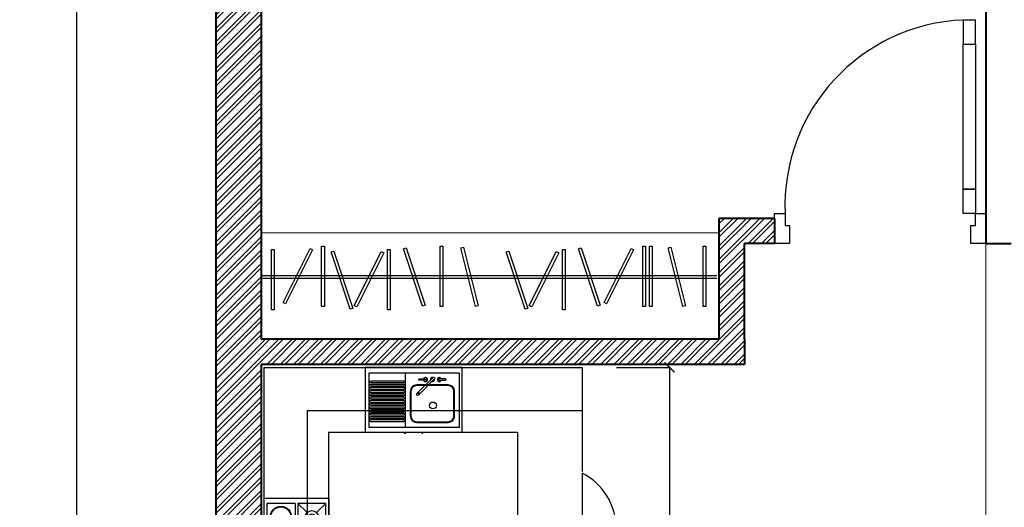
# Model space of a CAD drawing. Units: inches. Extents: x 528 to 2520, y -151 to 1354.
# Tile 30 of 41: x 2119 to 2315, y 635 to 731. Entities that reach past the tile are written whole.
import ezdxf

# ---------------------------------------------------------------- set-up
doc = ezdxf.new("R2010")
doc.units = ezdxf.units.IN
doc.header["$MEASUREMENT"] = 0
for name, color, linetype, lineweight in [('A-ANNO-DIMS', 2, 'Continuous', 18), ('A-Door', 150, 'Continuous', 25), ('A-ELEV-PROJ', 8, 'Continuous', 13), ('A-FLOR-CASE', 11, 'Continuous', 20), ('A-WALL-PATT', 6, 'Continuous', 13), ('walls', 7, 'Continuous', 40)]:
    doc.layers.add(name, color=color, linetype=linetype, lineweight=lineweight)
for name, color, linetype in [('ESYA', 11, 'Continuous'), ('HID', 11, 'Continuous'), ('NT', 1, 'Continuous'), ('TEFRIS', 11, 'Continuous')]:
    doc.layers.add(name, color=color, linetype=linetype)
doc.styles.get("Standard").update_dxf_attribs({"font": 'arial.ttf'})
doc.dimstyles.get("Standard").update_dxf_attribs({"dimtxt": 6, "dimasz": 2, "dimexe": 0.18, "dimexo": 0.0625, "dimgap": 0.09, "dimtad": 0, "dimtih": 1, "dimtoh": 1, "dimdec": 1, "dimzin": 0, "dimdsep": 46, "dimlunit": 3, "dimtxsty": 'Standard', "dimblk": 'ARCHTICK', "dimcen": 0.09, "dimadec": 0, "dimazin": 0, "dimtfac": 1, "dimtdec": 1, "dimtofl": 0, "dimtmove": 0, "dimatfit": 3, "dimfxl": 1, "dimtolj": 1, "dimtzin": 0, "dimarcsym": 0})

# ---------------------------------------------------------------- blocks, each defined once
blk = doc.blocks.new('A$C7DB75F4D')
at = {"layer": 'A-Door'}
for points in [[(625, 740), (625, 660), (665, 660), (665, 740)], [(625, 180), (625, 660), (665, 660), (665, 180)], [(625, 100), (625, 180), (665, 180), (665, 100)], [(35, 100), (35, 60), (50, 60), (50, 50), (50, 0), (0, 0), (0, 100)], [(665, 100), (700, 100), (700, 0), (650, 0), (650, 50), (650, 60), (665, 60)]]:
    blk.add_lwpolyline(points, close=True, dxfattribs=at)
at = {"layer": 'NT'}
blk.add_arc((650, 125), 615.5, 92.3278, 182.3278, dxfattribs=at)
blk = doc.blocks.new('A$C41BE763B')
at = {"layer": 'HID'}
for p, q in [((3.395, 0.2532), (0, 0.2532)), ((3.395, 0.2332), (0, 0.2332))]:
    blk.add_line(p, q, dxfattribs=at)
for points in [[(0.0983, 0.45), (0.0983, 0), (0.0775, 0), (0.0775, 0.45)], [(0.3834, 0.447), (0.1822, 0.0445), (0.1636, 0.0538), (0.3648, 0.4563)], [(0.4716, 0.4734), (0.4716, 0.0234), (0.4508, 0.0234), (0.4508, 0.4734)], [(0.9617, 0.45), (0.9617, 0), (0.941, 0), (0.941, 0.45)], [(1.0809, 0.4606), (1.2232, 0.0337), (1.2035, 0.0271), (1.0612, 0.454)], [(1.3547, 0.4734), (1.3547, 0.0234), (1.3339, 0.0234), (1.3339, 0.4734)], [(1.5084, 0.466), (1.6175, 0.0294), (1.5974, 0.0244), (1.4882, 0.4609)], [(2.2657, 0.45), (2.2657, 0), (2.2449, 0), (2.2449, 0.45)], [(2.3849, 0.4606), (2.5272, 0.0337), (2.5075, 0.0271), (2.3652, 0.454)], [(2.7757, 0.447), (2.5745, 0.0445), (2.5559, 0.0538), (2.7572, 0.4563)], [(2.8639, 0.4734), (2.8639, 0.0234), (2.8432, 0.0234), (2.8432, 0.4734)], [(2.9139, 0.4734), (2.9139, 0.0234), (2.8932, 0.0234), (2.8932, 0.4734)], [(3.0533, 0.466), (3.1624, 0.0294), (3.1423, 0.0244), (3.0332, 0.4609)], [(3.3139, 0.4734), (3.3139, 0.0234), (3.2932, 0.0234), (3.2932, 0.4734)], [(0.5408, 0.4372), (0.6831, 0.0103), (0.6634, 0.0037), (0.5211, 0.4306)], [(0.914, 0.4236), (0.7128, 0.0211), (0.6942, 0.0304), (0.8954, 0.4329)], [(1.8448, 0.4372), (1.9871, 0.0103), (1.9674, 0.0037), (1.8251, 0.4306)], [(2.218, 0.4236), (2.0167, 0.0211), (1.9981, 0.0304), (2.1994, 0.4329)]]:
    blk.add_lwpolyline(points, close=True, dxfattribs=at)
blk = doc.blocks.new('AR365L')
blk.add_line((0, 0.0995), (0.61, 0.0995))
blk.add_lwpolyline([(0, 0), (0, 0.68), (0.61, 0.68), (0.61, 0)], close=True)
blk = doc.blocks.new('FIRIN1')
at = {"layer": 'ESYA'}
for p, q in [((0.2875, -0.05), (0.2875, -0.3006)), ((0.3983, -0.1319), (0.3125, -0.05)), ((0.575, -0.05), (0.4892, -0.1319)), ((0.3983, -0.2187), (0.3125, -0.3006)), ((0.575, -0.3006), (0.4892, -0.2187)), ((0.2875, -0.3006), (0.025, -0.3006)), ((0.025, -0.3244), (0.1108, -0.4063)), ((0.2017, -0.4063), (0.2875, -0.3244)), ((0.3983, -0.4063), (0.3125, -0.3244)), ((0.575, -0.3244), (0.4892, -0.4063)), ((0.025, -0.575), (0.1108, -0.4931)), ((0.2017, -0.4931), (0.2875, -0.575)), ((0.3983, -0.4931), (0.3125, -0.575)), ((0.575, -0.575), (0.4892, -0.4931))]:
    blk.add_line(p, q, dxfattribs=at)
blk.add_lwpolyline([(0, 0), (0.6, 0), (0.6, -0.6), (0, -0.6)], close=True, dxfattribs=at)
for points in [[(0.2875, -0.05), (0.025, -0.05), (0.025, -0.3006)], [(0.3125, -0.05), (0.3125, -0.3006), (0.575, -0.3006)], [(0.575, -0.3006), (0.575, -0.05), (0.3125, -0.05)], [(0.2875, -0.575), (0.2875, -0.3244), (0.025, -0.3244)], [(0.025, -0.3244), (0.025, -0.575)], [(0.3125, -0.575), (0.3125, -0.3244), (0.575, -0.3244)], [(0.3125, -0.575), (0.575, -0.575), (0.575, -0.3244)], [(0.025, -0.575), (0.2875, -0.575)]]:
    blk.add_lwpolyline(points, dxfattribs=at)
for centre, radius in [((0.1562, -0.1753), 0.0986), ((0.1562, -0.1753), 0.0936), ((0.4438, -0.1753), 0.0597), ((0.4438, -0.1753), 0.0294), ((0.1562, -0.4497), 0.0492), ((0.1562, -0.4497), 0.0242), ((0.4438, -0.4497), 0.0398), ((0.4438, -0.4497), 0.0196)]:
    blk.add_circle(centre, radius, dxfattribs=at)
blk = doc.blocks.new('ncvn')
for p, q in [((77868.38, -4466.7), (77868.38, -4520.7)), ((77949.38, -4466.7), (77868.38, -4466.7)), ((77949.38, -4520.7), (77949.38, -4466.7))]:
    blk.add_line(p, q)
at = {"layer": 'TEFRIS'}
for p, q in [((77783.66, -4466.69), (77783.66, -4763.38)), ((77783.66, -4466.69), (78049.52, -4466.69)), ((78049.52, -4466.69), (78049.52, -4553.55)), ((77901.95, -4516.62), (77901.95, -4471.62)), ((77819.66, -4502.83), (77819.66, -4759.23)), ((77819.66, -4502.83), (78049.52, -4502.83)), ((77837.66, -4520.83), (77837.66, -4704.71)), ((77837.66, -4520.83), (77995.52, -4520.83)), ((77868.38, -4520.7), (77949.38, -4520.7)), ((77995.52, -4520.83), (77995.52, -4642.99)), ((78049.52, -4554.99), (78049.52, -4625.66)), ((78049.52, -4625.66), (77995.83, -4625.66)), ((77783.66, -4704.71), (77837.66, -4704.71))]:
    blk.add_line(p, q, dxfattribs=at)
for points in [[(77868.38, -4466.7), (77868.38, -4520.7), (77949.38, -4520.7), (77949.38, -4466.7)], [(77871.35, -4471.62), (77871.35, -4516.62), (77946.95, -4516.62), (77946.95, -4471.62)]]:
    blk.add_lwpolyline(points, close=True, dxfattribs=at)
for points in [[(77911.5, -4488.58), (77925.04, -4475.05, -1), (77926.25, -4476.26), (77912.72, -4489.8, -1)], [(77905.95, -4486.73), (77905.95, -4507.22, 0.414214), (77911.35, -4512.62), (77937.55, -4512.62, 0.414214), (77942.95, -4507.22), (77942.95, -4486.73, 0.414214), (77937.55, -4481.33), (77911.35, -4481.33, 0.414214)], [(77906.49, -4486.73), (77906.49, -4507.22, 0.414214), (77911.35, -4512.08), (77937.55, -4512.08, 0.414214), (77942.41, -4507.22), (77942.41, -4486.73, 0.414214), (77937.55, -4481.87), (77911.35, -4481.87, 0.414214)], [(77913.54, -4476.29), (77919.71, -4476.29, -0.563183), (77919.71, -4477.44), (77913.54, -4477.44, -1)], [(77935.33, -4476.29), (77929.17, -4476.29, 0.563183), (77929.17, -4477.44), (77935.33, -4477.44, 1)]]:
    blk.add_lwpolyline(points, format="xyb", close=True, dxfattribs=at)
for points in [[(77873.15, -4477.92), (77900.15, -4477.92, -1), (77900.15, -4479.72), (77873.15, -4479.72, -1), (77873.15, -4477.92)], [(77873.15, -4480.62), (77900.15, -4480.62, -1), (77900.15, -4482.42), (77873.15, -4482.42, -1), (77873.15, -4480.62)], [(77873.15, -4483.32), (77900.15, -4483.32, -1), (77900.15, -4485.12), (77873.15, -4485.12, -1), (77873.15, -4483.32)], [(77873.15, -4486.02), (77900.15, -4486.02, -1), (77900.15, -4487.82), (77873.15, -4487.82, -1), (77873.15, -4486.02)], [(77873.15, -4488.72), (77900.15, -4488.72, -1), (77900.15, -4490.52), (77873.15, -4490.52, -1), (77873.15, -4488.72)], [(77873.15, -4491.42), (77900.15, -4491.42, -1), (77900.15, -4493.22), (77873.15, -4493.22, -1), (77873.15, -4491.42)], [(77873.15, -4494.12), (77900.15, -4494.12, -1), (77900.15, -4495.92), (77873.15, -4495.92, -1), (77873.15, -4494.12)], [(77873.15, -4496.82), (77900.15, -4496.82, -1), (77900.15, -4498.62), (77873.15, -4498.62, -1), (77873.15, -4496.82)], [(77873.15, -4499.52), (77900.15, -4499.52, -1), (77900.15, -4501.32), (77873.15, -4501.32, -1), (77873.15, -4499.52)], [(77873.15, -4502.22), (77900.15, -4502.22, -1), (77900.15, -4504.02), (77873.15, -4504.02, -1), (77873.15, -4502.22)], [(77873.15, -4504.92), (77900.15, -4504.92, -1), (77900.15, -4506.72), (77873.15, -4506.72, -1), (77873.15, -4504.92)], [(77873.15, -4507.62), (77900.15, -4507.62, -1), (77900.15, -4509.42), (77873.15, -4509.42, -1), (77873.15, -4507.62)], [(77873.15, -4510.32), (77900.15, -4510.32, -1), (77900.15, -4512.12), (77873.15, -4512.12, -1), (77873.15, -4510.32)]]:
    blk.add_lwpolyline(points, format="xyb", dxfattribs=at)
for points in [[(77901.23, -4520.7), (77901.23, -4521.6), (77902.13, -4521.6), (77902.13, -4520.7)], [(77915.63, -4520.7), (77915.63, -4521.6), (77916.53, -4521.6), (77916.53, -4520.7)]]:
    blk.add_lwpolyline(points, dxfattribs=at)
for centre, radius in [((77913.01, -4488.3), 0.571), ((77924.89, -4498.48), 2.86)]:
    blk.add_circle(centre, radius, dxfattribs=at)
for centre, radius, start, end in [((77918.69, -4476.87), 1.71, 199.47122, 160.52878), ((77924.44, -4476.87), 1.71, 75, 195), ((77930.19, -4476.87), 1.71, 19.47122, 340.52878), ((77924.44, -4476.87), 1.71, 255, 15), ((78026.22, -4601.26), 51.8, 233.6588, 63.26709)]:
    blk.add_arc(centre, radius, start, end, dxfattribs=at)
at = {"layer": 'TEFRIS', "xscale": 90, "yscale": 90, "zscale": 90}
blk.add_blockref('FIRIN1', (77783.76, -4575.88), dxfattribs=at)
at = {"layer": 'TEFRIS', "xscale": 90, "yscale": 90, "zscale": 90, "rotation": 90}
blk.add_blockref('AR365L', (77848.22, -4760.91), dxfattribs=at)
blk = doc.blocks.new('_ArchTick')
at = {"color": 0, "linetype": 'ByBlock', "const_width": 0.15}
blk.add_lwpolyline([(-0.5, -0.5), (0.5, 0.5)], dxfattribs=at)
blk = doc.blocks.new('*D60')
at = {"layer": 'A-ANNO-DIMS', "color": 0, "lineweight": -2, "transparency": 16777216}
for p, q in [((2237.62, 662.36), (2248.32, 662.36)), ((2248.14, 662.36), (2248.14, 630.29)), ((2248.14, 591.82), (2248.14, 623.9)), ((2237.62, 591.82), (2248.32, 591.82))]:
    blk.add_line(p, q, dxfattribs=at)
at = {"layer": 'Defpoints', "color": 0, "transparency": 16777216}
for p in [(2237.56, 662.36), (2248.14, 662.36), (2237.56, 591.82)]:
    blk.add_point(p, dxfattribs=at)
at = {"layer": 'A-ANNO-DIMS', "color": 0, "lineweight": -2, "transparency": 16777216, "xscale": 2, "yscale": 2, "zscale": 2}
for p, rotation in [((2248.14, 662.36), 90), ((2248.14, 591.82), 270)]:
    blk.add_blockref('_ArchTick', p, dxfattribs=dict(at, rotation=rotation))
at = {"layer": 'A-ANNO-DIMS', "color": 0, "transparency": 16777216, "insert": (2248.14, 627.09), "char_height": 6, "attachment_point": 5}
blk.add_mtext('\\A1;KITCHEN COUNTER 5\'-10 1/2" TYP.', dxfattribs=at)
blk = doc.blocks.new('*D95')
at = {"layer": 'A-ANNO-DIMS', "color": 0, "lineweight": -2, "transparency": 16777216}
for p, q in [((2157.95, 897.94), (2130.18, 897.94)), ((2130.36, 897.94), (2130.36, 632.59)), ((2130.36, 360.94), (2130.36, 626.29)), ((2157.95, 360.94), (2130.18, 360.94))]:
    blk.add_line(p, q, dxfattribs=at)
at = {"layer": 'Defpoints', "color": 0, "transparency": 16777216}
for p in [(2130.36, 897.94), (2158.01, 897.94), (2158.01, 360.94)]:
    blk.add_point(p, dxfattribs=at)
at = {"layer": 'A-ANNO-DIMS', "color": 0, "lineweight": -2, "transparency": 16777216, "xscale": 2, "yscale": 2, "zscale": 2}
for p, rotation in [((2130.36, 897.94), 90), ((2130.36, 360.94), 270)]:
    blk.add_blockref('_ArchTick', p, dxfattribs=dict(at, rotation=rotation))
at = {"layer": 'A-ANNO-DIMS', "color": 0, "transparency": 16777216, "insert": (2130.36, 629.44), "char_height": 6, "attachment_point": 5}
blk.add_mtext('\\A1;44\'-9"', dxfattribs=at)

msp = doc.modelspace()

# ---------------------------------------------------------------- hatches: boundary and pattern name
at = {"layer": 'A-WALL-PATT'}
h = msp.add_hatch(dxfattribs=at)
h.set_pattern_fill('ANSI32', color=256, scale=5)
h.set_pattern_definition([(45, (1571.3155, -419.1643), (-1.3258252, 1.3258252), []), (45, (1572.1993, -419.1643), (-1.3258252, 1.3258252), [])])
h.paths.add_polyline_path([(2167.01, 744.69), (2158.01, 744.69), (2158.01, 549.94), (2169.56, 549.94), (2174.56, 549.94), (2174.56, 554.94), (2167.01, 554.94), (2167.01, 662.94), (2263.01, 662.94), (2263.01, 667.94), (2263.01, 686.94), (2269.01, 686.94), (2269.01, 691.94), (2258.01, 691.94), (2258.01, 667.94), (2167.01, 667.94)])
h.paths.add_polyline_path([(2260.02, 554.94), (2222.56, 554.94), (2222.56, 549.94), (2260.02, 549.94)])
h.paths.add_polyline_path([(2457.01, 752.2), (2448.01, 752.2), (2448.01, 691.94), (2358.01, 691.94), (2358.01, 686.94), (2448.01, 686.94), (2448.01, 554.94), (2358.01, 554.94), (2358.01, 549.94), (2448.01, 549.94), (2448.01, 405.94), (2406.01, 405.94), (2406.01, 396.94), (2457.01, 396.94)])
h.paths.add_polyline_path([(2457.01, 897.94), (2447.97, 897.94), (2447.97, 888.94), (2448.01, 888.94), (2448.01, 828.94), (2394.01, 828.94), (2394.01, 823.94), (2448.01, 823.94), (2448.01, 800.2), (2457.01, 800.2)])
h.paths.add_polyline_path([(2423.97, 897.94), (2359.01, 897.94), (2359.01, 828.94), (2355.58, 828.94), (2355.58, 823.94), (2364.01, 823.94), (2364.01, 829.94), (2364.01, 888.94), (2423.97, 888.94)])
h.paths.add_polyline_path([(2256.01, 897.94), (2191.01, 897.94), (2191.01, 888.94), (2251.01, 888.94), (2251.01, 828.94), (2251.01, 823.94), (2256.01, 823.94), (2256.01, 829.08)])
h.paths.add_polyline_path([(2167.01, 888.94), (2167.01, 897.94), (2158.01, 897.94), (2158.01, 792.69), (2167.01, 792.69), (2167.01, 823.94), (2221.01, 823.94), (2221.01, 828.94), (2167.01, 828.94)])
h.paths.add_polyline_path([(2316.01, 549.94), (2316.01, 554.94), (2296.02, 554.94), (2296.02, 549.94), (2311.01, 549.94), (2311.01, 455.12), (2316.01, 455.12)])
h.paths.add_polyline_path([(2311.01, 549.94), (2299.01, 549.94), (2299.01, 545.95), (2302.05, 545.95), (2302.05, 542.51), (2305.75, 542.51), (2305.75, 538.08), (2311.01, 538.08)], flags=17)
h.paths.add_polyline_path([(2358.01, 405.94), (2316.01, 405.94), (2316.01, 413.12), (2311.01, 413.12), (2311.01, 396.94), (2358.01, 396.94)])

# ---------------------------------------------------------------- linework, layer by layer
at = {"layer": 'A-ELEV-PROJ'}
for p, q in [((2158.01, 360.94), (2158.01, 897.94)), ((2311.01, 360.94), (2311.01, 897.94))]:
    msp.add_line(p, q, dxfattribs=at)
at = {"layer": 'A-FLOR-CASE'}
msp.add_line((2167.01, 689.1), (2258.01, 689.1), dxfattribs=at)
at = {"layer": 'walls'}
for p, q in [((2158.01, 897.94), (2158.01, 369.94)), ((2167.01, 823.94), (2167.01, 667.94)), ((2311.01, 823.94), (2311.01, 691.94)), ((2258.01, 667.94), (2258.01, 691.94)), ((2269.01, 691.94), (2258.01, 691.94)), ((2269.01, 691.94), (2269.01, 686.94)), ((2311.01, 691.94), (2311.01, 686.94)), ((2263.01, 667.94), (2263.01, 686.94)), ((2269.01, 686.94), (2263.01, 686.94)), ((2311.01, 686.94), (2316.01, 686.94)), ((2258.01, 667.94), (2167.01, 667.94)), ((2263.01, 667.94), (2263.01, 662.94)), ((2167.01, 662.94), (2167.01, 554.94)), ((2263.01, 662.94), (2167.01, 662.94))]:
    msp.add_line(p, q, dxfattribs=at)

# ---------------------------------------------------------------- block references
at = {"layer": 'A-Door', "xscale": 0.0600000000000059, "yscale": 0.0600000000000059, "zscale": 0.0600000000000059}
msp.add_blockref('A$C7DB75F4D', (2269.01, 686.94), dxfattribs=at)
at = {"layer": 'A-FLOR-CASE'}
for name, p, xscale, yscale, zscale in [('A$C41BE763B', (2167.01, 673.8), 26.66231123505322, 26.66231123505322, 26.66231123505322), ('ncvn', (-16325.27, 1724.3), 0.2377471155606993, 0.2377471155606993, 0.2377471155606993)]:
    msp.add_blockref(name, p, dxfattribs=dict(at, xscale=xscale, yscale=yscale, zscale=zscale))

# ---------------------------------------------------------------- dimensions: what is measured, and where the dimension line sits
at = {"layer": 'A-ANNO-DIMS'}
dim = msp.add_linear_dim(base=(2130.36, 897.94), p1=(2158.01, 360.94), p2=(2158.01, 897.94), angle=90, dimstyle='Standard', override={"dimdec": 1, "dimlfac": 1, "dimrnd": 0, "dimzin": 1, "dimdsep": 46, "dimlunit": 4, "dimfrac": 2}, dxfattribs=at)
dim.commit()
dim.dimension.update_dxf_attribs({"geometry": '*D95', "text_midpoint": (2130.36, 629.44)})
dim = msp.add_linear_dim(base=(2248.14, 662.36), p1=(2237.56, 591.82), p2=(2237.56, 662.36), angle=90, text='KITCHEN COUNTER <> TYP.', dimstyle='Standard', override={"dimdec": 1, "dimlfac": 1, "dimrnd": 0, "dimzin": 1, "dimdsep": 46, "dimlunit": 4, "dimfrac": 2}, dxfattribs=at)
dim.commit()
dim.dimension.update_dxf_attribs({"geometry": '*D60', "text_midpoint": (2248.14, 627.09)})

doc.saveas('drawing.dxf')
